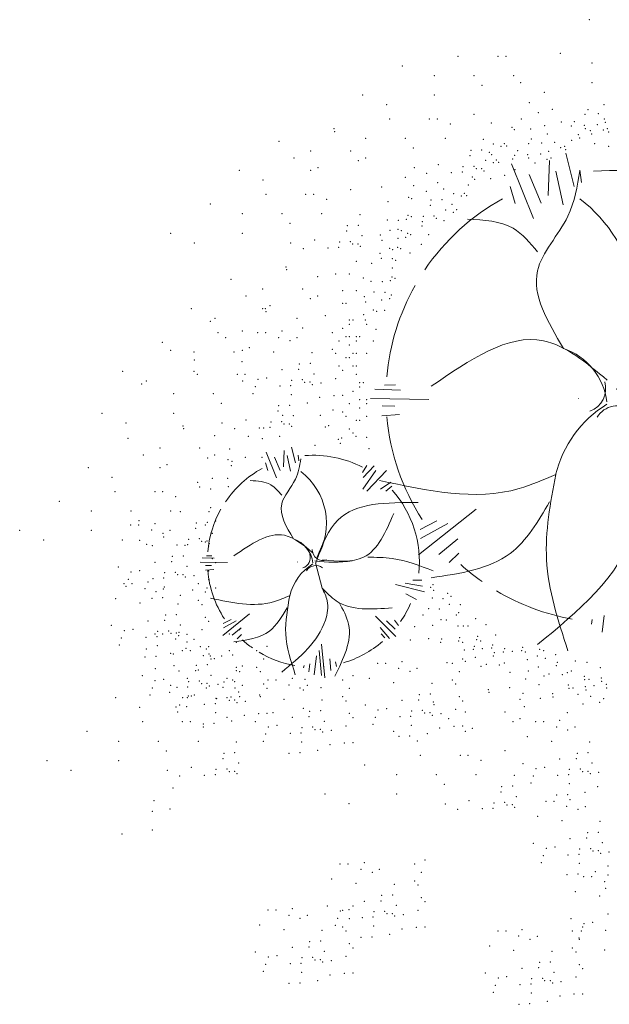
# Model space of a CAD drawing. Units: inches. Extents: x 1239 to 2276906, y 2273 to 321338.
# Tile 20 of 23: x 67865 to 67989, y 11321 to 11529. Entities that reach past the tile are written whole.
import ezdxf

# ---------------------------------------------------------------- set-up
doc = ezdxf.new("R2010")
doc.units = ezdxf.units.IN
doc.layers.add('L-PLNT', color=94, linetype='Continuous', lineweight=13)

# ---------------------------------------------------------------- blocks, each defined once
blk = doc.blocks.new('A$C30B31857')
for p, q in [((2.9834, 4.9924), (2.9378, 5.171)), ((2.7648, 4.82), (2.6466, 5.1137)), ((2.8434, 4.944), (2.8514, 5.1313)), ((2.8062, 4.9013), (2.7413, 5.0568)), ((2.9247, 4.894), (2.8853, 5.0751)), ((3.0223, 5.0135), (3.0144, 5.0799)), ((2.6661, 4.9009), (2.6393, 4.9915)), ((1.9621, 3.9222), (2.0223, 3.9241)), ((1.9103, 3.9012), (2.0497, 3.8956)), ((1.8883, 3.8498), (2.2022, 3.8449)), ((1.9494, 3.7571), (2.0441, 3.7647)), ((1.9499, 3.8105), (2.0188, 3.8098)), ((1.3819, 3.4241), (1.3265, 3.5618)), ((1.4188, 3.4822), (1.4225, 3.57)), ((1.4844, 3.5049), (1.463, 3.5887)), ((1.3356, 3.462), (1.3231, 3.5045)), ((1.4013, 3.4622), (1.3709, 3.5351)), ((1.4568, 3.4588), (1.4384, 3.5437)), ((1.5026, 3.5148), (1.4989, 3.546)), ((1.8439, 3.4518), (1.8684, 3.4899)), ((1.847, 3.3622), (1.9166, 3.4632)), ((1.8485, 3.4247), (1.9067, 3.4887)), ((1.868, 3.352), (1.973, 3.4627)), ((1.9418, 3.3622), (1.9966, 3.3999)), ((1.9699, 3.3518), (2.0024, 3.3789)), ((2.1467, 3.0086), (2.4563, 3.255)), ((2.1542, 3.1461), (2.2449, 3.1926)), ((2.1561, 3.097), (2.3032, 3.1772)), ((1.594, 2.9655), (1.6381, 3.0897)), ((2.2561, 3.01), (2.3583, 3.095)), ((0.971, 2.9694), (1.1182, 2.967)), ((0.9814, 2.9934), (1.0467, 2.9908)), ((1.0056, 3.0033), (1.0339, 3.0042)), ((2.3116, 2.9682), (2.3637, 3.0175)), ((0.9997, 2.9259), (1.0441, 2.9295)), ((0.9999, 2.9509), (1.0322, 2.9506)), ((1.5913, 2.9655), (1.6271, 2.8302)), ((2.1639, 2.8721), (2.1155, 2.8726)), ((2.1774, 2.8094), (2.0226, 2.8493)), ((2.1665, 2.8407), (2.0739, 2.8568)), ((2.1347, 2.7684), (2.0785, 2.7983)), ((1.0922, 2.575), (1.2373, 2.6905)), ((1.0957, 2.6395), (1.1382, 2.6613)), ((1.0966, 2.6164), (1.1655, 2.6541)), ((2.0239, 2.569), (1.9137, 2.6778)), ((2.0211, 2.6094), (1.9743, 2.6542)), ((2.0385, 2.6282), (2.0167, 2.6578)), ((3.0763, 2.6357), (3.0809, 2.6614)), ((3.1343, 2.5921), (3.1456, 2.6823)), ((1.1434, 2.5757), (1.1913, 2.6155)), ((1.9903, 2.5593), (1.9397, 2.6182)), ((1.1695, 2.5561), (1.1939, 2.5792)), ((1.9642, 2.5615), (1.9442, 2.5828)), ((1.6235, 2.359), (1.6107, 2.4933)), ((1.6415, 2.3458), (1.624, 2.5274)), ((1.584, 2.3634), (1.5971, 2.4652)), ((1.675, 2.3867), (1.6687, 2.4492)), ((1.5279, 2.4002), (1.5301, 2.4123)), ((1.5551, 2.3798), (1.5604, 2.4221)), ((1.7046, 2.4077), (1.6996, 2.4328))]:
    blk.add_line(p, q)
for centre, radius, start, end in [((3.1873, 3.861), 1.217, 62.402, 94.6709), ((3.1873, 3.861), 1.217, 118.935, 145.868), ((2.5377, 4.3028), 0.7844, 329.0782, 52.6009), ((3.1873, 3.861), 1.217, 150.5954, 174.9599), ((2.8122, 3.7899), 0.3494, 6.8841, 70.9351), ((3.0261, 3.9032), 0.1272, 289.2154, 17.1317), ((3.4797, 3.2971), 0.6129, 121.5433, 166.6017), ((3.1338, 3.8505), 0.1272, 179.4366, 180.2669), ((3.2157, 3.6838), 0.1272, 52.7337, 148.3189), ((3.1873, 3.861), 1.217, 185.1155, 212.961), ((1.58, 2.9746), 0.5705, 62.402, 94.6709), ((1.58, 2.9746), 0.5705, 118.935, 145.868), ((1.2979, 3.1775), 0.353, 329.0782, 52.6009), ((1.58, 2.9746), 0.5705, 353.5054, 42.0912), ((1.58, 2.9746), 0.5705, 150.5954, 174.9599), ((1.4214, 2.9466), 0.1572, 6.8841, 70.9351), ((1.633, 3.0374), 0.0596, 180.2669, 289.2154), ((1.5549, 2.9697), 0.0596, 179.4366, 180.2669), ((1.5044, 2.9943), 0.0596, 289.2154, 17.1317), ((1.6891, 3.6438), 0.6749, 261.4278, 278.5722), ((1.58, 2.9746), 0.5705, 185.1155, 212.961), ((1.7218, 2.7249), 0.2758, 121.5433, 166.6017), ((1.5933, 2.8915), 0.0596, 52.7337, 148.3189), ((3.1873, 3.861), 1.217, 227.9939, 234.9207), ((3.1873, 3.861), 1.217, 239.2549, 259.861), ((1.58, 2.9746), 0.5705, 325.3181, 336.4192), ((1.58, 2.9746), 0.5705, 227.9939, 234.9207), ((1.58, 2.9746), 0.5705, 286.5005, 310.702), ((1.58, 2.9746), 0.5705, 239.2549, 259.861)]:
    blk.add_arc(centre, radius, start, end)
for points, knots in [([(2.9263, 4.1201), (2.841, 4.2637), (2.6905, 4.5171), (2.9681, 4.7985), (3.0006, 4.9937), (3.0146, 5.0775)], [0, 0, 0, 0, 0.440566, 0.777274, 1.031196, 1.031196, 1.031196, 1.031196]), ([(2.7862, 4.6403), (2.7459, 4.6888), (2.6503, 4.8039), (2.4983, 4.8115), (2.4103, 4.8158)], [0, 0, 0, 0, 0.1819315, 0.4317682, 0.4317682, 0.4317682, 0.4317682]), ([(3.1616, 3.9488), (3.0492, 4.0429), (2.7553, 4.2891), (2.4209, 4.0585), (2.2144, 3.9161)], [0, 0, 0, 0, 0.40354, 1.055721, 1.055721, 1.055721, 1.055721]), ([(1.4728, 3.0952), (1.4344, 3.1599), (1.3667, 3.2739), (1.4916, 3.4005), (1.5062, 3.4883), (1.5125, 3.5261)], [0, 0, 0, 0, 0.1982546, 0.3497731, 0.4640382, 0.4640382, 0.4640382, 0.4640382]), ([(3.2693, 3.5312), (3.2945, 3.4812), (3.355, 3.361), (3.2868, 2.9371), (3.0051, 2.7057), (2.786, 2.5256)], [0, 0, 0, 0, 0.165135, 0.396758, 1.208872, 1.208872, 1.208872, 1.208872]), ([(1.4097, 3.3293), (1.3916, 3.3512), (1.3486, 3.403), (1.2802, 3.4063), (1.2406, 3.4083)], [0, 0, 0, 0, 0.0818692, 0.1942957, 0.1942957, 0.1942957, 0.1942957]), ([(2.884, 3.4417), (2.819, 3.4131), (2.522, 3.2824), (2.1934, 3.3535), (1.9367, 3.409)], [0, 0, 0, 0, 0.2107352, 0.9627078, 0.9627078, 0.9627078, 0.9627078]), ([(2.884, 3.4417), (2.8554, 3.2883), (2.7956, 2.967), (2.8966, 2.6556), (2.9493, 2.4929)], [0, 0, 0, 0, 0.4606481, 0.9645387, 0.9645387, 0.9645387, 0.9645387]), ([(1.6007, 2.9961), (1.6311, 3.0708), (1.7211, 3.2914), (1.9759, 3.2909), (2.1445, 3.2905)], [0, 0, 0, 0, 0.2272785, 0.6713114, 0.6713114, 0.6713114, 0.6713114]), ([(2.8513, 3.2945), (2.7895, 3.1889), (2.6492, 2.9493), (2.3704, 2.9084), (2.2144, 2.8855)], [0, 0, 0, 0, 0.3498703, 0.7941952, 0.7941952, 0.7941952, 0.7941952]), ([(1.6301, 2.9813), (1.7105, 2.9741), (1.8949, 2.9574), (1.9699, 3.1328), (2.0122, 3.2316)], [0, 0, 0, 0, 0.2209637, 0.5066723, 0.5066723, 0.5066723, 0.5066723]), ([(1.5786, 3.0182), (1.5281, 3.0605), (1.3958, 3.1713), (1.2454, 3.0675), (1.1524, 3.0034)], [0, 0, 0, 0, 0.1815929, 0.4750743, 0.4750743, 0.4750743, 0.4750743]), ([(1.8726, 2.9961), (1.917, 2.9955), (2.0386, 2.9939), (2.1529, 2.9502), (2.2254, 2.9225)], [0, 0, 0, 0, 0.132489, 0.3627011, 0.3627011, 0.3627011, 0.3627011]), ([(1.6271, 2.8302), (1.6384, 2.8077), (1.6657, 2.7536), (1.635, 2.5629), (1.5082, 2.4587), (1.4096, 2.3777)], [0, 0, 0, 0, 0.0743107, 0.1785413, 0.5439924, 0.5439924, 0.5439924, 0.5439924]), ([(1.6271, 2.8302), (1.6515, 2.8046), (1.7474, 2.7036), (1.8949, 2.7151), (2.0049, 2.7237)], [0, 0, 0, 0, 0.1034892, 0.4070428, 0.4070428, 0.4070428, 0.4070428]), ([(1.4537, 2.79), (1.4245, 2.7771), (1.2909, 2.7183), (1.143, 2.7503), (1.0275, 2.7752)], [0, 0, 0, 0, 0.0948308, 0.4332185, 0.4332185, 0.4332185, 0.4332185]), ([(1.4537, 2.79), (1.4409, 2.7209), (1.414, 2.5763), (1.4594, 2.4362), (1.4831, 2.363)], [0, 0, 0, 0, 0.2072917, 0.4340424, 0.4340424, 0.4340424, 0.4340424]), ([(1.439, 2.7237), (1.4112, 2.6762), (1.3481, 2.5684), (1.2226, 2.55), (1.1524, 2.5397)], [0, 0, 0, 0, 0.1574416, 0.3573878, 0.3573878, 0.3573878, 0.3573878]), ([(1.7183, 2.7531), (1.7397, 2.7142), (1.8095, 2.5877), (1.7426, 2.4506), (1.6962, 2.3556)], [0, 0, 0, 0, 0.1285246, 0.4177469, 0.4177469, 0.4177469, 0.4177469])]:
    blk.add_open_spline(points, degree=3, knots=knots)
for p in [(3.0641, 5.8899), (2.3591, 5.6932), (2.573, 5.6932), (2.6157, 5.6932), (2.9089, 5.7085), (2.0597, 5.641), (3.08, 5.6562), (2.2308, 5.5888), (2.4447, 5.5888), (2.6585, 5.5888), (2.4874, 5.5365), (2.695, 5.5518), (3.08, 5.5518), (1.8458, 5.4843), (2.2308, 5.4843), (2.8233, 5.4996), (1.9741, 5.4321), (2.7419, 5.4438), (3.1439, 5.4325), (1.99, 5.3551), (2.2039, 5.3551), (2.2466, 5.3551), (2.4447, 5.3798), (2.6996, 5.3561), (2.7913, 5.389), (2.8662, 5.4068), (3.0424, 5.3801), (3.0582, 5.4047), (3.1125, 5.3835), (3.1453, 5.3553), (1.6906, 5.3028), (2.3163, 5.3276), (2.5373, 5.3341), (2.6493, 5.3108), (2.749, 5.3012), (2.8239, 5.319), (2.9138, 5.3383), (2.9681, 5.3172), (2.9838, 5.3417), (3.0381, 5.3205), (3.0438, 5.303), (3.1081, 5.3239), (3.151, 5.3378), (3.1624, 5.3027), (1.6946, 5.2876), (1.8617, 5.2506), (2.0755, 5.2506), (2.2894, 5.2506), (2.6617, 5.2971), (2.8395, 5.2754), (3.0066, 5.2715), (3.0123, 5.2539), (3.071, 5.2924), (3.0767, 5.2748), (3.141, 5.2957), (3.1681, 5.2851), (1.3952, 5.2354), (2.1183, 5.1984), (2.495, 5.2464), (2.5488, 5.2203), (2.5903, 5.208), (2.607, 5.223), (2.607, 5.223), (2.6194, 5.2093), (2.738, 5.223), (2.7537, 5.2475), (2.808, 5.2263), (2.878, 5.2297), (2.9109, 5.2015), (2.9323, 5.2085), (2.9323, 5.2085), (2.9695, 5.24), (3.0938, 5.2222), (3.1695, 5.208), (1.4767, 5.1462), (1.5663, 5.1831), (1.7801, 5.1831), (1.8617, 5.1462), (2.4236, 5.1572), (2.428, 5.186), (2.4862, 5.1888), (2.5277, 5.1764), (2.54, 5.1627), (2.6636, 5.16), (2.6794, 5.1845), (2.7336, 5.1634), (2.7393, 5.1458), (2.8037, 5.1667), (2.8465, 5.1806), (2.8579, 5.1455), (2.938, 5.191), (1.605, 5.0939), (1.8229, 5.1309), (2.1231, 5.0932), (2.2518, 5.1099), (2.3857, 5.0983), (2.4439, 5.101), (2.5065, 5.1325), (2.548, 5.1202), (2.5647, 5.1353), (2.5771, 5.1216), (2.652, 5.1394), (2.7722, 5.1177), (2.8365, 5.1386), (1.1813, 5.0787), (1.5663, 5.0787), (2.0755, 5.0417), (2.1906, 5.0632), (2.3231, 5.0667), (2.3813, 5.0695), (2.4351, 5.0434), (2.4562, 5.0873), (2.4853, 5.0887), (2.4977, 5.0749), (2.6097, 5.0516), (2.665, 5.0828), (1.3096, 5.0264), (1.9472, 4.9895), (2.1202, 4.9958), (2.2488, 5.0125), (2.4139, 4.9995), (2.4474, 5.0297), (2.5347, 5.0338), (1.3255, 4.9494), (1.5393, 4.9494), (1.5821, 4.9494), (1.7801, 4.9742), (2.0927, 4.934), (2.1876, 4.9658), (2.2808, 4.979), (2.3346, 4.9529), (2.376, 4.9406), (2.3928, 4.9556), (2.3928, 4.9556), (2.4051, 4.9419), (1.0261, 4.8972), (1.6518, 4.922), (1.9809, 4.9098), (2.1095, 4.9265), (2.2094, 4.8898), (2.2138, 4.9186), (2.272, 4.9214), (2.3258, 4.8953), (1.1972, 4.845), (1.411, 4.845), (1.6249, 4.845), (1.8305, 4.8407), (2.0897, 4.8366), (2.0897, 4.8366), (2.1066, 4.8291), (2.1715, 4.8309), (2.2297, 4.8336), (2.2923, 4.8651), (2.3337, 4.8528), (2.3505, 4.8679), (1.4538, 4.7928), (1.7635, 4.7804), (1.8217, 4.7831), (1.9779, 4.8124), (2.0376, 4.8104), (2.0805, 4.816), (2.1648, 4.7785), (2.167, 4.8021), (2.242, 4.8199), (2.2835, 4.8075), (0.8122, 4.7405), (1.1972, 4.7405), (1.7591, 4.7516), (1.842, 4.7269), (1.9412, 4.73), (1.9933, 4.7562), (2.0362, 4.7618), (2.053, 4.7542), (2.0776, 4.7186), (2.0868, 4.7392), (2.1036, 4.7317), (2.1997, 4.7321), (0.9405, 4.6883), (1.4586, 4.6875), (1.5873, 4.7043), (1.7212, 4.6926), (1.7794, 4.6954), (1.7917, 4.6817), (1.8208, 4.683), (1.8332, 4.6693), (1.9489, 4.7019), (2.0347, 4.7131), (2.1619, 4.6811), (1.526, 4.6575), (1.6586, 4.6611), (1.7168, 4.6638), (1.9383, 4.6326), (1.9903, 4.6588), (2.0072, 4.6513), (2.0332, 4.6644), (2.0501, 4.6569), (2.1007, 4.6343), (1.4322, 4.5592), (1.8112, 4.5888), (1.8939, 4.5783), (1.946, 4.6045), (2.0057, 4.6026), (2.0226, 4.5951), (1.4362, 4.5439), (1.6032, 4.507), (1.7005, 4.5212), (1.7743, 4.5212), (2.0042, 4.5539), (1.1367, 4.4917), (1.8481, 4.4986), (1.8909, 4.4809), (1.9507, 4.479), (1.9936, 4.4846), (2.0028, 4.5052), (2.0028, 4.5052), (2.0196, 4.4977), (1.2183, 4.4025), (1.3078, 4.4395), (1.5217, 4.4395), (1.6032, 4.4025), (1.7374, 4.431), (1.8112, 4.431), (1.9063, 4.4247), (1.9661, 4.4228), (1.9998, 4.4078), (1.3466, 4.3503), (1.5645, 4.3872), (1.7374, 4.3634), (1.7558, 4.3634), (1.8543, 4.3986), (1.862, 4.3705), (1.9477, 4.3816), (1.9906, 4.3872), (0.9229, 4.335), (1.3078, 4.335), (1.3214, 4.3338), (1.3254, 4.3186), (1.6451, 4.2957), (1.8513, 4.3012), (1.9034, 4.3274), (1.9202, 4.3199), (1.9631, 4.3254), (1.026, 4.2664), (1.0512, 4.2828), (1.4925, 4.2816), (1.7743, 4.2732), (1.7743, 4.2732), (1.7743, 4.2506), (1.7928, 4.2732), (1.859, 4.2731), (1.8666, 4.2506), (1.0671, 4.2058), (1.1971, 4.2141), (1.2809, 4.2058), (1.3237, 4.2058), (1.411, 4.2141), (1.5217, 4.2306), (1.682, 4.2056), (1.7374, 4.2281), (1.9173, 4.2225), (0.7676, 4.1536), (1.1075, 4.1772), (1.3934, 4.1783), (1.4537, 4.1619), (1.4925, 4.1772), (1.7189, 4.1605), (1.7558, 4.183), (1.7743, 4.183), (1.7743, 4.1379), (1.8112, 4.183), (1.8112, 4.1605), (1.8297, 4.183), (1.9035, 4.1605), (0.8121, 4.1097), (0.9387, 4.1013), (1.1526, 4.1013), (1.1971, 4.1097), (1.2359, 4.1249), (1.3665, 4.1013), (1.5721, 4.0971), (1.682, 4.1154), (1.7005, 4.0929), (1.7928, 4.0929), (1.8112, 4.0929), (1.8666, 4.0929), (0.9404, 4.0574), (1.1954, 4.0491), (1.5051, 4.0368), (1.5633, 4.0395), (1.7558, 4.0703), (1.7743, 4.0703), (0.5538, 3.9969), (0.9387, 3.9969), (0.9563, 3.9804), (1.1702, 3.9804), (1.2129, 3.9804), (1.411, 4.0052), (1.5007, 4.008), (1.5836, 3.9833), (1.7189, 4.0252), (1.7374, 4.0027), (1.7928, 4.0252), (1.8112, 4.0252), (1.8112, 3.9801), (0.6569, 3.9282), (0.6821, 3.9447), (1.2002, 3.9439), (1.2826, 3.953), (1.3289, 3.9606), (1.4628, 3.949), (1.521, 3.9517), (1.5333, 3.938), (1.5624, 3.9394), (1.5748, 3.9257), (1.6207, 3.9335), (1.7005, 3.9576), (1.8297, 3.9351), (1.8297, 3.9351), (1.8481, 3.9351), (0.828, 3.876), (1.0418, 3.876), (1.2557, 3.876), (1.2676, 3.9139), (1.4001, 3.9175), (1.4583, 3.9202), (1.4613, 3.8717), (1.7928, 3.89), (1.8297, 3.9125), (1.0846, 3.8238), (1.547, 3.8267), (1.6145, 3.8567), (1.6911, 3.8661), (1.7374, 3.8674), (1.7743, 3.8223), (1.8297, 3.8449), (1.8666, 3.8449), (1.8666, 3.8223), (0.443, 3.7715), (0.828, 3.7715), (1.3899, 3.7826), (1.3943, 3.8114), (1.4525, 3.8141), (1.6849, 3.7894), (1.7374, 3.7773), (1.8297, 3.7998), (0.5713, 3.7193), (1.0894, 3.7186), (1.2181, 3.7353), (1.352, 3.7236), (1.4102, 3.7264), (1.4147, 3.7591), (1.4226, 3.7127), (1.4517, 3.714), (1.4728, 3.7579), (1.6174, 3.7593), (1.7558, 3.7547), (1.8112, 3.7322), (1.8297, 3.7322), (1.8666, 3.7547), (0.8784, 3.7029), (0.8824, 3.6876), (1.1569, 3.6885), (1.2894, 3.6921), (1.3136, 3.6915), (1.3476, 3.6948), (1.464, 3.7003), (1.6449, 3.6975), (1.6618, 3.7051), (1.7743, 3.6871), (1.7928, 3.6645), (0.583, 3.6354), (1.0495, 3.6506), (1.2301, 3.6464), (1.3048, 3.6339), (1.3994, 3.6464), (1.7153, 3.6302), (1.7153, 3.6302), (1.7245, 3.6096), (1.7322, 3.6377), (1.8088, 3.6471), (1.8666, 3.642), (0.7541, 3.5832), (0.9679, 3.5832), (1.1291, 3.5788), (1.5881, 3.5982), (1.8792, 3.5798), (0.6645, 3.5462), (1.0107, 3.5309), (1.0495, 3.5462), (1.1203, 3.5212), (1.1417, 3.5118), (1.2148, 3.5337), (1.304, 3.5338), (0.3691, 3.4787), (0.7541, 3.4787), (0.7928, 3.494), (1.1379, 3.4887), (0.4974, 3.4265), (0.9571, 3.3992), (1.0368, 3.4211), (1.1194, 3.4211), (0.5133, 3.3495), (0.7272, 3.3495), (0.7699, 3.3495), (0.9679, 3.3742), (1.028, 3.3635), (1.1225, 3.376), (0.2139, 3.2972), (0.8396, 3.322), (0.385, 3.245), (0.5988, 3.245), (0.8127, 3.245), (0.8648, 3.2414), (1.0183, 3.2408), (1.0271, 3.2633), (0.6416, 3.1928), (1.0095, 3.1832), (1.0544, 3.1915), (0, 3.1406), (0.385, 3.1406), (0.5979, 3.1692), (0.6407, 3.1692), (0.7104, 3.1417), (0.728, 3.1775), (0.8095, 3.1406), (0.9469, 3.1516), (0.9513, 3.1804), (0.999, 3.169), (0.1283, 3.0883), (0.5529, 3.0883), (0.6464, 3.0876), (0.7708, 3.1253), (0.7751, 3.1043), (0.909, 3.0927), (0.9672, 3.0954), (0.9795, 3.0817), (0.999, 3.0788), (1.0086, 3.0831), (1.0298, 3.1269), (1.036, 3.1239), (0.6835, 3.0647), (0.7139, 3.0576), (0.8464, 3.0611), (0.8891, 3.0605), (0.9046, 3.0639), (1.0175, 3.0562), (1.021, 3.0693), (0.728, 2.9686), (0.8177, 2.9714), (0.8221, 3.0002), (0.8803, 3.0029), (1.036, 2.9886), (0.53, 2.9438), (0.5997, 2.9164), (0.6459, 2.924), (0.9006, 2.9467), (1.0175, 2.921), (1.0544, 2.9661), (0.5846, 2.8773), (0.7172, 2.8809), (0.7754, 2.8836), (0.7798, 2.9124), (0.838, 2.9151), (0.8503, 2.9014), (0.8794, 2.9028), (0.8918, 2.8891), (0.9377, 2.8969), (1.0175, 2.876), (0.561, 2.8537), (0.5727, 2.8394), (0.6038, 2.8537), (0.6735, 2.8262), (0.6911, 2.862), (0.7338, 2.8098), (0.7726, 2.8251), (0.7783, 2.8351), (0.9315, 2.8201), (0.9621, 2.8535), (1.0081, 2.8295), (1.0544, 2.8308), (2.2113, 2.8337), (2.2113, 2.8337), (2.2237, 2.8474), (2.2281, 2.8186), (0.516, 2.7728), (0.7113, 2.7748), (0.7695, 2.7775), (0.864, 2.7901), (0.9621, 2.7633), (0.999, 2.8084), (2.2201, 2.7761), (2.2783, 2.7733), (2.303, 2.8008), (2.3198, 2.7857), (0.6466, 2.7492), (0.8522, 2.745), (0.9806, 2.7408), (2.1998, 2.7198), (2.258, 2.7171), (2.3118, 2.7432), (2.37, 2.7404), (0.6911, 2.6531), (0.7808, 2.6559), (0.7852, 2.6847), (0.8434, 2.6874), (0.999, 2.6731), (1.0175, 2.6506), (2.1698, 2.6846), (2.2668, 2.6595), (2.2959, 2.6581), (2.3497, 2.6842), (2.3621, 2.6979), (2.4538, 2.665), (0.4931, 2.6284), (0.5627, 2.6009), (0.609, 2.6086), (0.8011, 2.5996), (0.8637, 2.6312), (0.9806, 2.6055), (1.1836, 2.6056), (2.1255, 2.6213), (2.2227, 2.6286), (2.3585, 2.6266), (2.3876, 2.6252), (2.4113, 2.6255), (2.5085, 2.6327), (0.5477, 2.5618), (0.6803, 2.5654), (0.7272, 2.5833), (0.7385, 2.5681), (0.7429, 2.5969), (0.7699, 2.5833), (0.8134, 2.5859), (0.8396, 2.5558), (0.8425, 2.5873), (0.8549, 2.5736), (0.8572, 2.5916), (0.9008, 2.5814), (0.9387, 2.5547), (1.1283, 2.5831), (2.1027, 2.5511), (2.1999, 2.5584), (2.2699, 2.555), (2.3614, 2.5447), (2.3614, 2.5447), (2.3671, 2.5623), (2.4585, 2.5519), (2.4642, 2.5695), (2.48, 2.545), (2.5614, 2.5767), (0.5358, 2.5239), (0.6821, 2.5024), (0.7414, 2.5197), (0.8748, 2.4932), (0.8946, 2.5046), (0.9, 2.5394), (0.9176, 2.4932), (0.9712, 2.5141), (1.0049, 2.5015), (1.0175, 2.5153), (1.1283, 2.4929), (1.1652, 2.538), (1.2759, 2.4929), (1.3313, 2.5155), (2.2642, 2.5375), (2.3828, 2.5377), (2.3928, 2.4957), (2.4414, 2.4993), (2.4471, 2.5168), (2.49, 2.5029), (2.5386, 2.5065), (2.5443, 2.5241), (2.6086, 2.5032), (2.7001, 2.4929), (2.7001, 2.4929), (2.7058, 2.5104), (2.7972, 2.5001), (2.8187, 2.4931), (0.6744, 2.4593), (0.7326, 2.4621), (0.8127, 2.4788), (0.8271, 2.4746), (0.9873, 2.4657), (1.0183, 2.4746), (1.0261, 2.4635), (1.0301, 2.4482), (1.0476, 2.4493), (1.0864, 2.4645), (1.1467, 2.4703), (1.3128, 2.4478), (2.3834, 2.4479), (2.4514, 2.4572), (2.5486, 2.4645), (2.5543, 2.482), (2.6029, 2.4856), (2.6515, 2.4892), (2.7215, 2.4859), (2.7315, 2.4438), (2.7858, 2.465), (2.8287, 2.4511), (2.883, 2.4722), (0.7307, 2.396), (0.8298, 2.4123), (0.9469, 2.3855), (0.9513, 2.4143), (0.9604, 2.3887), (1.0095, 2.417), (1.1652, 2.4027), (1.1972, 2.4112), (1.2759, 2.4027), (1.6362, 2.407), (1.927, 2.4255), (1.9698, 2.4255), (2.0394, 2.3981), (2.057, 2.4339), (2.1386, 2.3969), (2.3, 2.4288), (2.3281, 2.4253), (2.3972, 2.436), (2.4829, 2.4082), (2.5101, 2.4188), (2.5801, 2.4154), (2.6072, 2.426), (2.7901, 2.4054), (2.8873, 2.4126), (2.893, 2.4302), (2.9902, 2.4374), (3.0533, 2.4302), (3.1244, 2.4005), (0.6592, 2.3579), (0.7751, 2.3381), (0.8572, 2.3827), (0.9017, 2.3437), (1.0298, 2.3608), (1.1156, 2.3437), (1.1467, 2.3351), (1.166, 2.3844), (1.1836, 2.3802), (1.2944, 2.3802), (1.3363, 2.3354), (1.3791, 2.3354), (1.4663, 2.3437), (1.5352, 2.3394), (1.7374, 2.3352), (1.7928, 2.3577), (1.8819, 2.3447), (2.0998, 2.3816), (2.3281, 2.3351), (2.365, 2.3802), (2.6387, 2.377), (2.7228, 2.3398), (2.7359, 2.3842), (2.8216, 2.3563), (2.8488, 2.3669), (2.9188, 2.3636), (2.9459, 2.3742), (2.9674, 2.384), (3.0386, 2.3544), (3.0405, 2.336), (3.0629, 2.3384), (3.1302, 2.3455), (0.7139, 2.2914), (0.7289, 2.3305), (0.8122, 2.3068), (0.8464, 2.2949), (0.9046, 2.2977), (0.909, 2.3265), (0.9672, 2.3292), (0.9795, 2.3155), (1.0049, 2.2926), (1.0086, 2.3169), (1.021, 2.3032), (1.0669, 2.311), (1.0946, 2.2953), (1.099, 2.3241), (1.1572, 2.3268), (1.1584, 2.2915), (1.1972, 2.3068), (1.3128, 2.3126), (1.3313, 2.29), (1.4488, 2.3079), (1.5091, 2.2915), (1.5263, 2.2818), (1.5479, 2.3068), (1.6209, 2.2943), (1.7743, 2.2901), (2.0125, 2.3211), (2.2181, 2.3168), (2.3465, 2.3126), (2.5212, 2.2832), (2.6369, 2.2936), (2.7939, 2.3101), (2.9527, 2.3083), (2.9547, 2.2899), (2.9547, 2.2899), (2.9771, 2.2923), (3.0443, 2.2993), (3.0463, 2.281), (3.0892, 2.3041), (3.1321, 2.3271), (3.1564, 2.3111), (3.1584, 2.2928), (0.5168, 2.2393), (0.702, 2.2535), (0.8069, 2.2678), (0.8765, 2.2403), (0.9017, 2.2393), (0.9076, 2.2492), (0.9228, 2.248), (0.9405, 2.2545), (1.0567, 2.2363), (1.0607, 2.2342), (1.1149, 2.2391), (1.1373, 2.2436), (1.1563, 2.2267), (1.1775, 2.2706), (1.1836, 2.2449), (1.2912, 2.2545), (1.2944, 2.2449), (1.4218, 2.2309), (1.6274, 2.2267), (1.7374, 2.245), (2.1467, 2.2277), (2.1511, 2.2565), (2.2093, 2.2592), (2.365, 2.245), (2.5252, 2.2679), (2.6923, 2.2309), (2.7081, 2.264), (2.8016, 2.2367), (2.8669, 2.2621), (2.8689, 2.2438), (3.0034, 2.2579), (3.0726, 2.2466), (3.1417, 2.2353), (0.6451, 2.1871), (0.8405, 2.1889), (0.8615, 2.2012), (0.8987, 2.1916), (0.9933, 2.2042), (0.9941, 2.2048), (1.0523, 2.2075), (1.1272, 2.2254), (1.1687, 2.213), (1.2146, 2.2209), (1.5255, 2.1817), (1.7559, 2.2225), (1.859, 2.2002), (1.9749, 2.1804), (2.057, 2.225), (2.2258, 2.2157), (2.2296, 2.203), (2.3465, 2.1773), (2.3834, 2.2224), (2.7158, 2.1906), (3.0316, 2.2052), (3.1213, 2.2146), (0.8496, 2.1633), (1.0552, 2.1591), (1.1156, 2.1348), (1.2084, 2.1441), (1.285, 2.1535), (1.3313, 2.1548), (1.3632, 2.1597), (1.4663, 2.1348), (1.556, 2.1376), (1.5604, 2.1664), (1.6186, 2.1691), (1.7743, 2.1548), (1.7928, 2.1323), (1.9137, 2.1336), (1.9287, 2.1727), (2.0462, 2.1372), (2.1044, 2.1399), (2.1088, 2.1687), (2.167, 2.1715), (2.1794, 2.1578), (2.2085, 2.1591), (2.2208, 2.1454), (2.2667, 2.1533), (2.3074, 2.1265), (2.3969, 2.1635), (2.6108, 2.1635), (2.6923, 2.1265), (2.9458, 2.1591), (0.661, 2.1101), (0.8748, 2.1101), (0.9176, 2.1101), (0.9873, 2.0826), (0.9882, 2.0988), (1.0464, 2.1015), (1.1409, 2.114), (1.2683, 2.1101), (1.338, 2.0826), (1.3842, 2.0903), (1.5181, 2.0786), (1.5763, 2.0813), (1.5887, 2.0676), (1.6178, 2.069), (1.6389, 2.1129), (1.7559, 2.0872), (1.9018, 2.0957), (2.1074, 2.0915), (2.2605, 2.0765), (2.3371, 2.0859), (2.3834, 2.0872), (2.4357, 2.0743), (2.6536, 2.1112), (2.7761, 2.1101), (2.8189, 2.1101), (2.8886, 2.0826), (2.9061, 2.1184), (2.9877, 2.0814), (0.3615, 2.0578), (1.323, 2.0435), (1.4555, 2.0471), (1.5137, 2.0498), (1.6301, 2.0553), (1.6761, 2.0631), (2.0119, 2.059), (2.0404, 2.0312), (2.0986, 2.0339), (2.1931, 2.0464), (2.3969, 2.059), (2.731, 2.0292), (2.9489, 2.0662), (0.5326, 2.0056), (0.7465, 2.0056), (0.9604, 2.0056), (1.166, 2.0014), (1.3111, 2.0056), (1.5167, 2.0014), (1.6698, 1.9863), (1.7464, 1.9958), (1.7928, 1.997), (2.1403, 2.0068), (2.8616, 2.0056), (3.0672, 2.0014), (0.7893, 1.9534), (1.0946, 1.9122), (1.099, 1.941), (1.1572, 1.9438), (1.4497, 1.941), (1.5079, 1.9438), (1.6024, 1.9563), (2.1561, 1.9298), (2.37, 1.9298), (2.4128, 1.9298), (2.6108, 1.9545), (2.9061, 1.9095), (2.9958, 1.9122), (3.0002, 1.941), (3.0584, 1.9438), (0.1477, 1.9011), (0.5326, 1.9011), (0.9228, 1.8649), (1.1149, 1.856), (1.1775, 1.8875), (1.8567, 1.8776), (2.4825, 1.9023), (2.7081, 1.8847), (2.7778, 1.8572), (2.824, 1.8649), (3.0161, 1.856), (3.0787, 1.8875), (0.276, 1.8489), (0.7941, 1.8482), (0.8615, 1.8181), (0.9941, 1.8217), (1.0523, 1.8245), (1.0567, 1.8533), (1.1272, 1.8423), (1.1563, 1.8436), (1.1687, 1.8299), (2.0278, 1.8253), (2.2417, 1.8253), (2.4555, 1.8253), (2.6611, 1.8211), (2.7628, 1.8181), (2.8953, 1.8217), (2.9535, 1.8245), (2.9579, 1.8533), (3.0285, 1.8423), (3.0576, 1.8436), (3.0699, 1.8299), (3.1158, 1.8378), (0.8241, 1.7535), (2.2844, 1.7731), (2.5941, 1.7607), (2.6523, 1.7635), (2.7509, 1.7803), (2.9565, 1.776), (3.1096, 1.761), (1.6428, 1.7209), (2.0278, 1.7209), (2.5897, 1.7319), (2.6726, 1.7072), (2.8895, 1.7157), (2.9477, 1.7184), (3.0422, 1.731), (0.723, 1.6859), (1.7712, 1.6686), (2.2893, 1.6679), (2.4179, 1.6846), (2.5474, 1.6442), (2.5518, 1.673), (2.61, 1.6757), (2.6224, 1.662), (2.6515, 1.6634), (2.6638, 1.6497), (2.8315, 1.6819), (2.8742, 1.6819), (2.9439, 1.6544), (2.9615, 1.6902), (3.043, 1.6533), (0.7142, 1.6283), (0.8087, 1.6408), (2.3567, 1.6379), (2.4892, 1.6414), (2.7864, 1.601), (3.0043, 1.638), (2.917, 1.5774), (3.1226, 1.5732), (0.551, 1.5062), (0.7133, 1.5282), (3.0556, 1.5129), (3.1138, 1.5156), (2.7635, 1.4565), (2.8794, 1.4367), (2.9615, 1.4813), (3.0512, 1.4841), (3.1341, 1.4594), (2.8182, 1.39), (2.8332, 1.4291), (2.9507, 1.3936), (3.0089, 1.3963), (3.0133, 1.4251), (3.0715, 1.4278), (3.0838, 1.4141), (3.1129, 1.4155), (3.1253, 1.4018), (3.1712, 1.4096), (1.7239, 1.3439), (1.7667, 1.3439), (1.854, 1.3522), (2.125, 1.3436), (2.1804, 1.3662), (2.8063, 1.3521), (3.0119, 1.3478), (3.165, 1.3328), (1.8364, 1.3164), (1.8967, 1.3), (1.9355, 1.3152), (2.1619, 1.2986), (2.9448, 1.2875), (3.0031, 1.2902), (3.0345, 1.2763), (3.0773, 1.2763), (3.0976, 1.3028), (3.1645, 1.2846), (1.6789, 1.263), (1.8095, 1.2394), (2.0151, 1.2352), (2.125, 1.2535), (2.1435, 1.2309), (3.147, 1.2488), (1.9481, 1.1748), (2.0063, 1.1776), (2.9894, 1.1954), (3.1201, 1.1718), (3.1537, 1.2133), (1.656, 1.1185), (1.7928, 1.1183), (1.854, 1.1433), (1.9437, 1.146), (2.0266, 1.1213), (2.1619, 1.1633), (2.1804, 1.1408), (1.3363, 1.096), (1.3791, 1.096), (1.4488, 1.0685), (1.4663, 1.1043), (1.5479, 1.0674), (1.7256, 1.0911), (1.7374, 1.0958), (1.7719, 1.0987), (1.9058, 1.0871), (1.964, 1.0898), (1.9763, 1.0761), (2.0054, 1.0775), (2.0178, 1.0637), (2.0637, 1.0716), (2.1435, 1.0957), (3.1645, 1.0757), (1.2912, 1.0151), (1.5091, 1.0521), (1.6987, 1.0141), (1.7106, 1.052), (1.7743, 1.0507), (1.8432, 1.0555), (1.9014, 1.0583), (1.9043, 1.0098), (2.9665, 1.0509), (3.0362, 1.0235), (3.0824, 1.0311), (1.4218, 0.9915), (1.6274, 0.9873), (1.7374, 1.0056), (1.7559, 0.983), (1.99, 0.9648), (2.0575, 0.9948), (2.1341, 1.0042), (2.1804, 1.0055), (2.573, 0.9833), (2.6158, 0.9833), (2.6855, 0.9559), (2.7031, 0.9916), (2.7846, 0.9547), (2.9741, 0.9831), (3.0212, 0.9843), (3.0295, 1.0056), (3.1537, 0.9879), (1.5604, 0.927), (1.6186, 0.9297), (1.7743, 0.9154), (1.8373, 0.9495), (1.8955, 0.9522), (2.528, 0.9024), (2.7459, 0.9394), (3.0093, 0.9465), (3.011, 0.938), (1.2683, 0.8706), (1.3842, 0.8508), (1.4663, 0.8954), (1.556, 0.8982), (1.6389, 0.8735), (1.7928, 0.8929), (2.6586, 0.8789), (2.8642, 0.8746), (2.9741, 0.8929), (2.9926, 0.8704), (3.1479, 0.8819), (1.323, 0.8041), (1.338, 0.8432), (1.4555, 0.8076), (1.5137, 0.8104), (1.5181, 0.8392), (1.5763, 0.8419), (1.5887, 0.8282), (1.6178, 0.8296), (1.6301, 0.8159), (1.6761, 0.8237), (1.7559, 0.8478), (2.7972, 0.8143), (2.8554, 0.817), (3.011, 0.8027), (1.3111, 0.7662), (1.5167, 0.7619), (1.6698, 0.7469), (1.7464, 0.7563), (1.7928, 0.7576), (2.5051, 0.758), (2.7031, 0.7827), (2.7928, 0.7855), (2.8757, 0.7608), (3.0295, 0.7802), (1.4497, 0.7016), (1.5079, 0.7043), (1.6024, 0.7169), (2.5597, 0.6914), (2.5748, 0.7305), (2.621, 0.7382), (2.6923, 0.695), (2.7505, 0.6977), (2.7549, 0.7265), (2.8131, 0.7293), (2.8254, 0.7155), (2.8545, 0.7169), (2.8669, 0.7032), (2.9128, 0.711), (2.9926, 0.7351), (2.5478, 0.6535), (2.7534, 0.6493), (2.9832, 0.6437), (3.0295, 0.6449), (2.6864, 0.5889), (2.7446, 0.5917), (2.8391, 0.6042), (2.9066, 0.6342)]:
    blk.add_point(p)
blk = doc.blocks.new('p2')
at = {"xscale": 1000, "yscale": 1000, "zscale": 1000}
blk.add_blockref('A$C30B31857', (-714.2, -1628.3), dxfattribs=at)

msp = doc.modelspace()

# ---------------------------------------------------------------- block references
at = {"layer": 'L-PLNT', "xscale": 0.0393700787401575, "yscale": 0.0393700787401575, "zscale": 0.0393700787401575}
msp.add_blockref('p2', (67892.66, 11361.51), dxfattribs=at)

doc.saveas('drawing.dxf')
